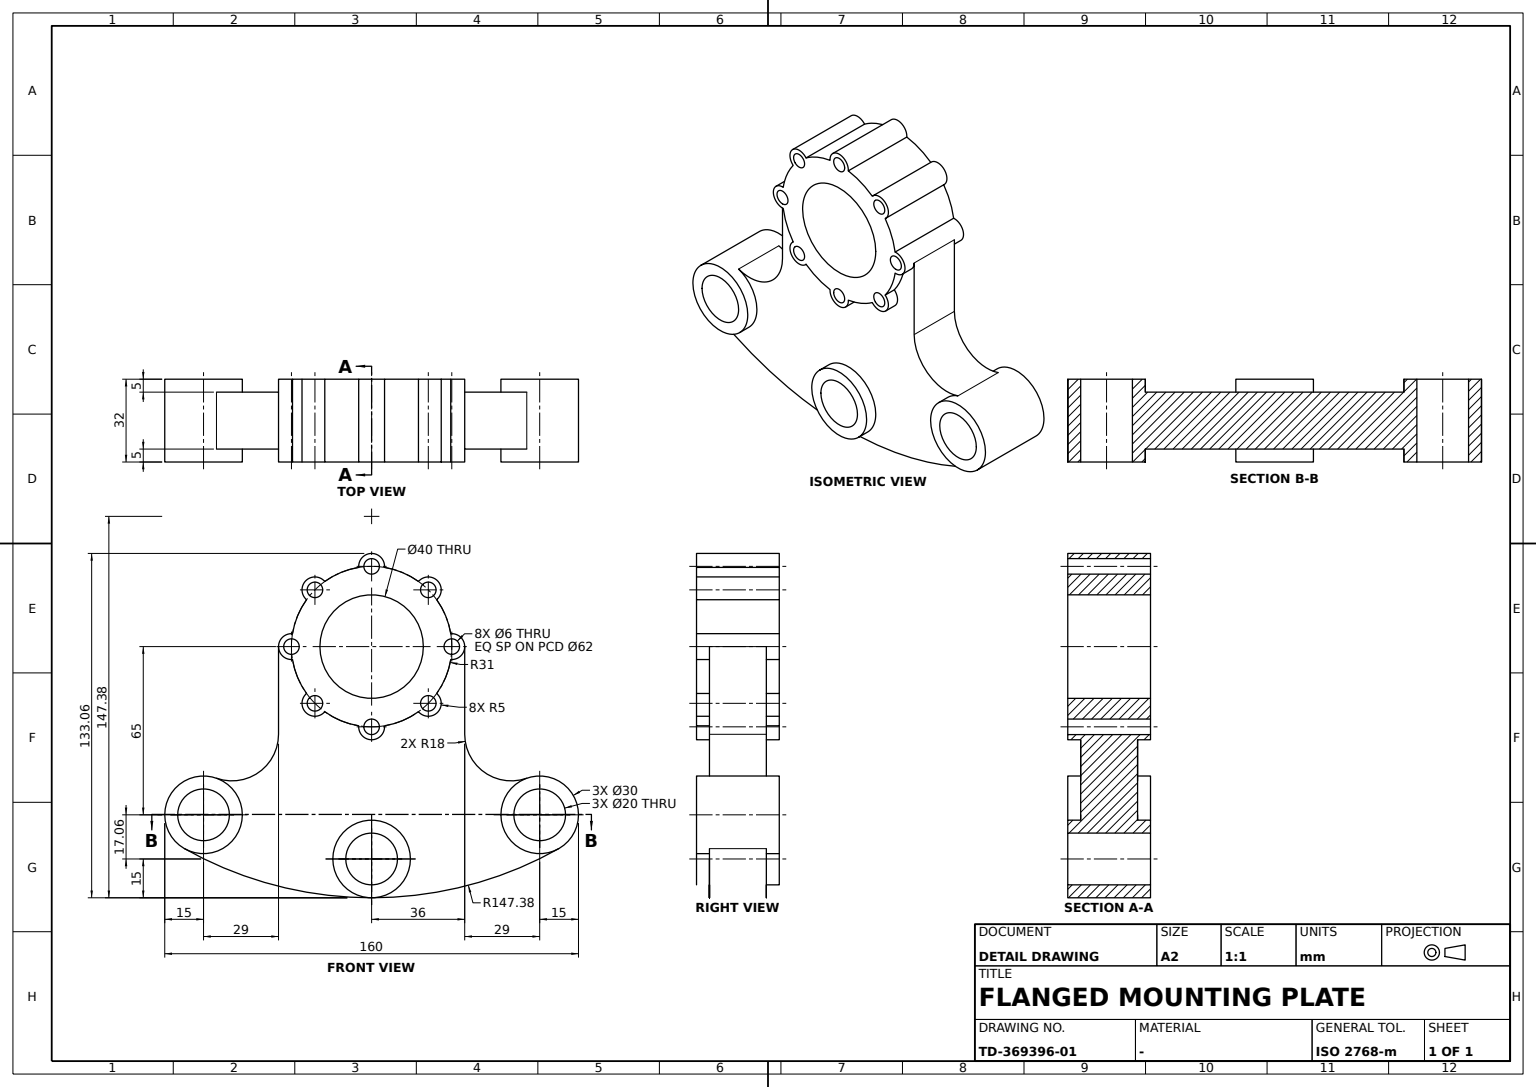
CATIA V5 part; units mm, degrees
sketch "Sketch1" plane through (0, 0, 0) normal (1, 0, 0) x (0, 1, 0)
  point P0 (-31, 0)
  point P1 (31, 0)
  circle A0 centre (0, 0) radius 31
  circle A1 centre (0, 0) radius 20
  dimension "radius A0" = 31
  dimension "radius A1" = 20
  constraint coincidence P0 x-axis
  constraint coincidence P1 A0
  constraint coincidence P0 A0
extrude "Pad1" add sketch "Sketch1" along normal mid plane 32
sketch "Sketch2" plane through (16, 0, 0) normal (1, 0, 0) x (0, 1, 0)
  circle A0 centre (0, 0) radius 31 construction
  circle A1 centre (0, 31) radius 5
  point P0 (0, 31)
  dimension "radius A1" = 5
  constraint coincidence P0 A0
  constraint coincidence P0 y-axis
extrude "Pad2" add sketch "Sketch2" against normal blind 32
sketch "Sketch3" plane through (16, 0, 0) normal (1, 0, 0) x (0, 1, 0)
  circle A0 centre (0, 31) radius 3
  point P0 (0, 31)
  point P1 (0, 28)
  dimension "radius A0" = 3
  dimension "distance origin P0" = 31
  constraint coincidence P0 y-axis
  constraint coincidence A0 P1
  constraint coincidence P1 y-axis
extrude "Pocket1" cut sketch "Sketch3" against normal blind 32
pattern_circular "CircPattern1" count 8 over 360 about axis through (16, 0, 0) along (1, 0, 0) of "Pad2", "Pocket1"
sketch "Sketch4" plane through (0, 0, 0) normal (1, 0, 0) x (0, 1, 0)
  circle A0 centre (0, -82.057) radius 15
  point P0 (0, -82.057)
  circle A1 centre (0, -82.057) radius 10
  circle A2 centre (65, -65) radius 15
  point P1 (65, -65)
  circle A3 centre (65, -65) radius 10
  circle A4 centre (-65, -65) radius 10
  circle A5 centre (-65, -65) radius 15
  dimension "radius A1" = 10
  dimension "radius A0" = 15
  dimension "distance P1 P0 x axis" = 65
  dimension "distance origin P1 y axis" = 65
  dimension "distance origin P0" = 82.057
  constraint coincidence P0 y-axis
  constraint equal size A1 A3
  constraint equal size A0 A2
  constraint symmetry A3 A4 y-axis
  constraint symmetry A2 A5 y-axis
extrude "Pad3" add sketch "Sketch4" along normal mid plane 32
sketch "Sketch5" plane through (0, 0, 0) normal (1, 0, 0) x (0, 1, 0)
  circle A0 centre (-65, -65) radius 15 construction
  arc A1 (-60, -50.8579) -> (-72.3653, -78.0672) centre (-65, -65) ccw
  circle A2 centre (65, -65) radius 15 construction
  arc A3 (72.3653, -78.0672) -> (60, -50.8579) centre (65, -65) ccw
  arc A4 (-72.3653, -78.0672) -> (72.3653, -78.0672) centre (0, 50.321) ccw
  point P0 (0, 50.321)
  circle A5 centre (0, -82.057) radius 15 construction
  point P1 (72.3653, -78.0672)
  point P2 (-72.3653, -78.0672)
  point P3 (-36, 0)
  line L0 (-36, 0) -> (-36, -33.8873)
  circle A6 centre (-31, 0) radius 5 construction
  arc A7 (-36, -33.8873) -> (-60, -50.8579) centre (-54, -33.8873) cw
  point P4 (-36, -33.8873)
  point P5 (-60, -50.8579)
  point P6 (60, -50.8579)
  point P7 (36, -33.8873)
  arc A8 (36, -33.8873) -> (60, -50.8579) centre (54, -33.8873) ccw
  point P8 (36, 0)
  line L1 (36, 0) -> (36, -33.8873)
  dimension "radius A7" = 18
  constraint coincidence P0 y-axis
  constraint coincidence A2 P1
  constraint coincidence A0 P2
  constraint coincidence P3 x-axis
  constraint coincidence P3 A6
  constraint tangency A4 A2
  constraint tangency A4 A5
  constraint tangency A7 L0
  constraint tangency A7 A0
  constraint vertical L0 y-axis
  constraint symmetry P5 P6 y-axis
  constraint symmetry P4 P7 y-axis
  constraint symmetry A7 A8 y-axis
  constraint symmetry P3 P8 y-axis
  constraint symmetry L0 L1 y-axis
extrude "Pad4" add sketch "Sketch5" along normal mid plane 22 material side at (0, -35.95, -16.9437)
equation "\"angular step@CircPattern1\" = 360.0*1 deg/CircPattern1.AngularNumber"
properties part number "Flanged Mounting Plate with Three Mounting Lugs"
